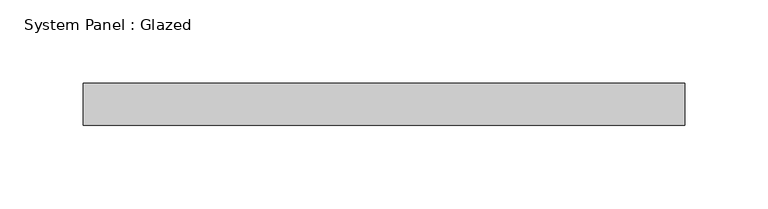
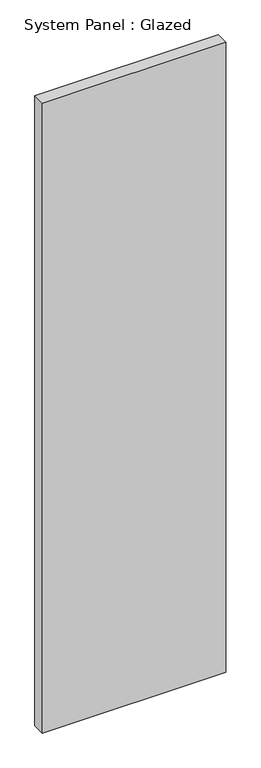
"""IFC4 building model written with IfcOpenShell, lengths in millimetres: plate geometry, System Panel : Glazed."""

from ifc_helpers import new_model, si_unit, origin, origin_with_axes, place, context, project, spatial, polyline, outline, extrude, source, transform, mapped, element, save


def system_panel_glazed_5760ca47(model_context):
    return source(origin(), model_context, "Body", "SweptSolid", [
        extrude(outline(polyline([(180.975, 19.05), (-180.975, 19.05), (-180.975, 44.45), (180.975, 44.45), (180.975, 19.05)])), origin_with_axes(), (0.0, 0.0, 1.0), 1314.7145247),
    ])


if __name__ == "__main__":
    model = new_model("IFC4")
    model_context = context("Model", 3, world=origin())
    ifc_project = project(units=[si_unit("LENGTHUNIT", "METRE", prefix="MILLI")], contexts=[model_context])
    site = spatial("IfcSite", under=ifc_project)
    building = spatial("IfcBuilding", under=site)
    placement = place(None, origin())
    system_panel_glazed_shape = system_panel_glazed_5760ca47(model_context)
    element("IfcPlate", 1, ObjectType="System Panel : Glazed", at=placement, inside=building, context=model_context, shape_type="MappedRepresentation", body=[
        mapped(system_panel_glazed_shape, transform((0.0, 0.0, 0.0), x_axis=(1.0, 0.0, 0.0), y_axis=(0.0, 1.0, 0.0), z_axis=(0.0, 0.0, 1.0))),
    ])
    save(model, "model.ifc")

# Revit data of these elements
# Type "System Panel : Glazed"
#   Construction Type Id = "GSP4R"
#   Analytic Construction = "1/8 in Pilkington single glazing"
#   Visual Light Transmittance = 0.9
#   Solar Heat Gain Coefficient = 0.86
#   Heat Transfer Coefficient (U) = 1.18115 BTU/(h·ft²·°F)
#   Define Thermal Properties by = 1
# Element 1 (IfcPlate, "System Panel : Glazed")
#   Materials on its faces: "Glass"
# Materials
#   "Glass": class "Glass", colour RGB 0 128 192, transparency 0.75, Description = "Soda Lime Glass", Cost = 0
